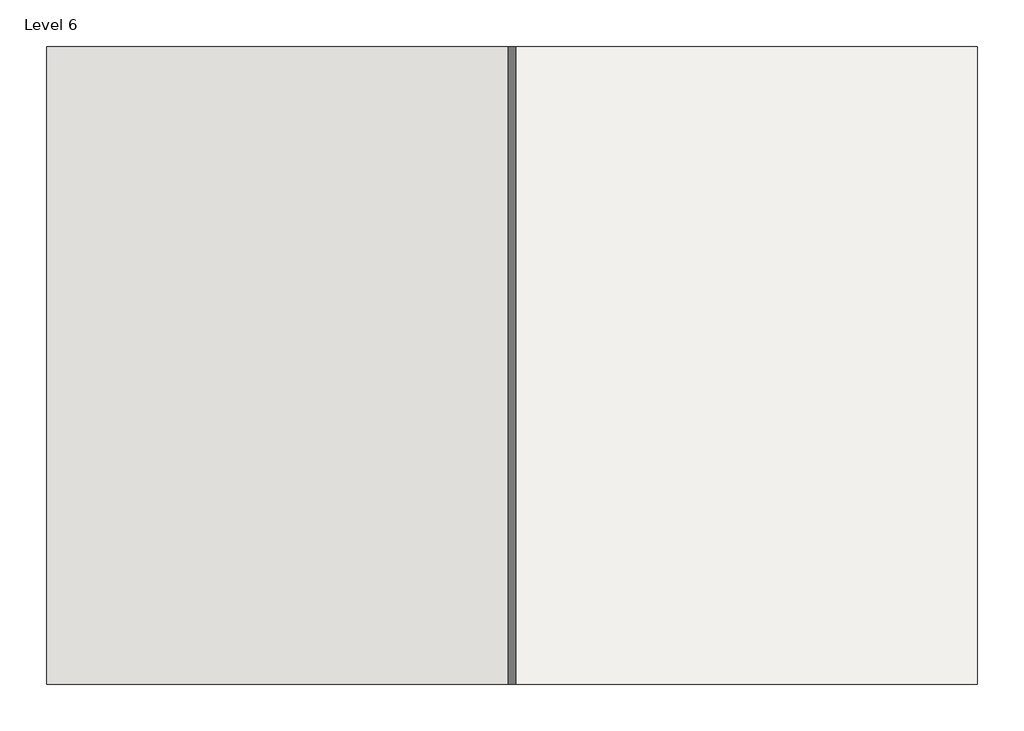
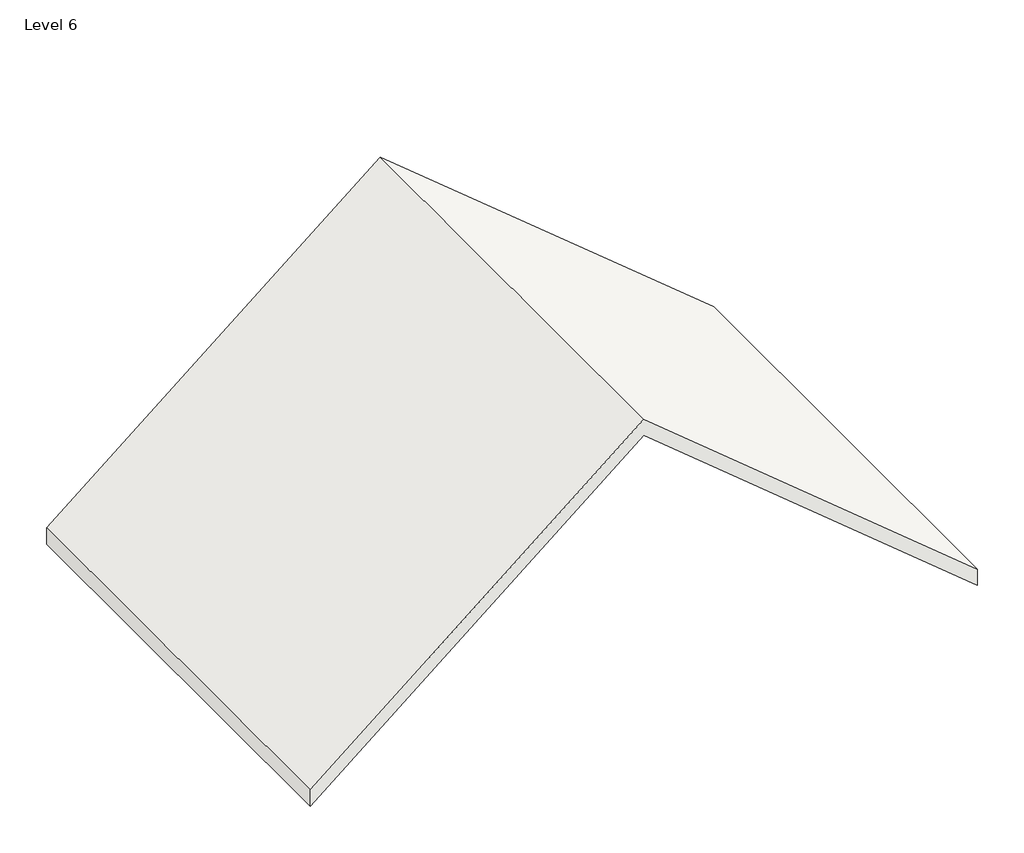
# One storey: 1 roof.
"""IFC4 building model written with IfcOpenShell, lengths in millimetres."""

from ifc_helpers import new_model, si_unit, frame, origin, place, context, project, spatial, polyline, outline, extrude, element, save

model = new_model("IFC4")

# Units and contexts
model_context = context("Model", 3, world=origin())
ifc_project = project(units=[si_unit("LENGTHUNIT", "METRE", prefix="MILLI")], contexts=[model_context])

# Site, building, storey
site = spatial("IfcSite", under=ifc_project)
building = spatial("IfcBuilding", under=site)
storey = spatial("IfcBuildingStorey", under=building, Name="Level 6", Elevation=7620.0)

# Roof
placement = place(None, origin())
element("IfcRoof", 1, ObjectType="6\"", at=placement, inside=storey, context=model_context, shape_type="SweptSolid", body=[
    extrude(outline(polyline([(6737.2622494, -5486.2332364), (6605.5234441, -5486.2332364), (8707.4611946, -2939.6548078), (6605.5234441, -393.0763793), (6737.2622494, -393.0763793), (8839.2, -2939.6548078), (6737.2622494, -5486.2332364)])), frame((0.0, -783.5961605, 0.0), z_axis=(0.0, 1.0, 0.0), x_axis=(0.0, 0.0, 1.0)), (0.0, 0.0, 1.0), 3488.4575887),
])

save(model, "model.ifc")

# Revit data of these elements
# Type "6\""
#   Assembly Code = "B1020"
#   Layers, outside or top first: 0' - 4" "roof" (function 1)
# Element 1 (IfcRoof, "6\"")
#   built-in parameter 1001710 = 33615
#   Phase Created = New Construction
#   Materials on its faces: "roof"
# Materials
#   "roof": class "Generic", colour RGB 120 120 120, transparency 0, Cost = 0
